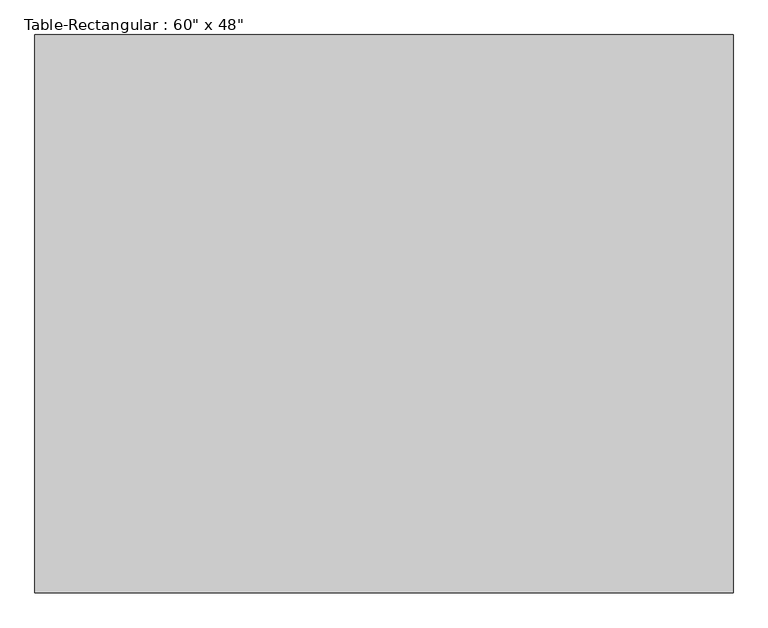
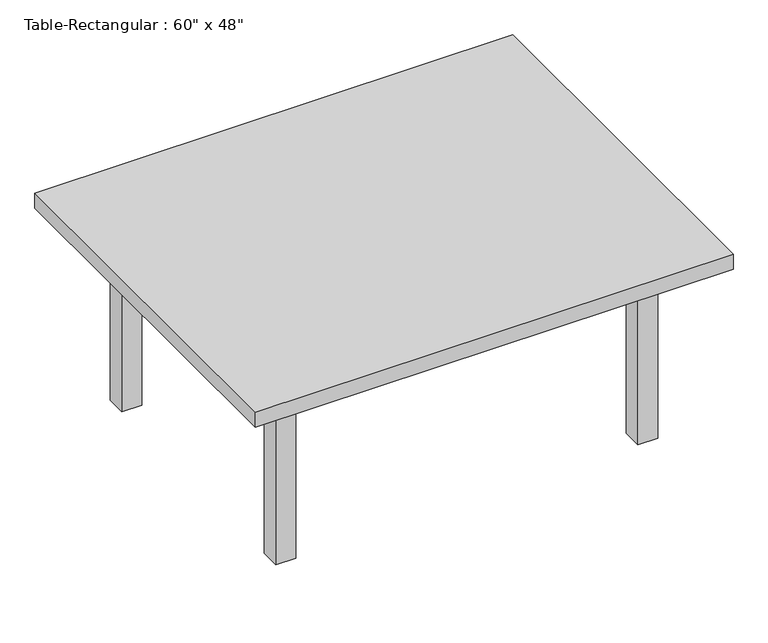
"""IFC4 building model written with IfcOpenShell, lengths in millimetres: furniture geometry."""

from ifc_helpers import new_model, si_unit, frame, origin, origin_with_axes, place, context, project, spatial, polyline, outline, extrude, source, transform, mapped, element, save


def furniture_e8434c74(model_context):
    return source(origin(), model_context, "Body", "SweptSolid", [
        extrude(outline(polyline([(546.1, 419.1), (546.1, 393.7), (-546.1, 393.7), (-546.1, 419.1), (546.1, 419.1)])), frame((0.0, 0.0, 508.0), z_axis=(0.0, 0.0, 1.0), x_axis=(1.0, 0.0, 0.0)), (0.0, 0.0, 1.0), 101.6),
        extrude(outline(polyline([(546.1, -419.1), (-546.1, -419.1), (-546.1, -393.7), (546.1, -393.7), (546.1, -419.1)])), frame((0.0, 0.0, 508.0), z_axis=(0.0, 0.0, 1.0), x_axis=(1.0, 0.0, 0.0)), (0.0, 0.0, 1.0), 101.6),
        extrude(outline(polyline([(-558.8, -393.7), (-584.2, -393.7), (-584.2, 393.7), (-558.8, 393.7), (-558.8, -393.7)])), frame((0.0, 0.0, 508.0), z_axis=(0.0, 0.0, 1.0), x_axis=(1.0, 0.0, 0.0)), (0.0, 0.0, 1.0), 101.6),
        extrude(outline(polyline([(558.8, -393.7), (558.8, 393.7), (584.2, 393.7), (584.2, -393.7), (558.8, -393.7)])), frame((0.0, 0.0, 508.0), z_axis=(0.0, 0.0, 1.0), x_axis=(1.0, 0.0, 0.0)), (0.0, 0.0, 1.0), 101.6),
        extrude(outline(polyline([(762.0, 609.6), (762.0, -609.6), (-762.0, -609.6), (-762.0, 609.6), (762.0, 609.6)])), frame((0.0, 0.0, 609.6), z_axis=(0.0, 0.0, 1.0), x_axis=(1.0, 0.0, 0.0)), (0.0, 0.0, 1.0), 50.8),
        extrude(outline(polyline([(-546.1, 457.2), (-546.1, 393.7), (-609.6, 393.7), (-609.6, 457.2), (-546.1, 457.2)])), origin_with_axes(), (0.0, 0.0, 1.0), 609.6),
        extrude(outline(polyline([(546.1, 457.2), (609.6, 457.2), (609.6, 393.7), (546.1, 393.7), (546.1, 457.2)])), origin_with_axes(), (0.0, 0.0, 1.0), 609.6),
        extrude(outline(polyline([(-546.1, -457.2), (-609.6, -457.2), (-609.6, -393.7), (-546.1, -393.7), (-546.1, -457.2)])), origin_with_axes(), (0.0, 0.0, 1.0), 609.6),
        extrude(outline(polyline([(546.1, -457.2), (546.1, -393.7), (609.6, -393.7), (609.6, -457.2), (546.1, -457.2)])), origin_with_axes(), (0.0, 0.0, 1.0), 609.6),
    ])


if __name__ == "__main__":
    model = new_model("IFC4")
    model_context = context("Model", 3, world=origin())
    ifc_project = project(units=[si_unit("LENGTHUNIT", "METRE", prefix="MILLI")], contexts=[model_context])
    site = spatial("IfcSite", under=ifc_project)
    building = spatial("IfcBuilding", under=site)
    placement = place(None, origin())
    furniture_shape = furniture_e8434c74(model_context)
    element("IfcFurniture", 1, ObjectType="Table-Rectangular : 60\" x 48\"", at=placement, inside=building, context=model_context, shape_type="MappedRepresentation", body=[
        mapped(furniture_shape, transform((0.0, 0.0, 0.0), x_axis=(1.0, 0.0, 0.0), y_axis=(0.0, 1.0, 0.0), z_axis=(0.0, 0.0, 1.0))),
    ])
    save(model, "model.ifc")

# Revit data of these elements
# Type "Table-Rectangular : 60\" x 48\""
#   Assembly Code = "E2020200"
#   Height = 2' - 2"
#   Length = 5' - 0"
#   Width = 4' - 0"
#   Base Material = Birch
#   Top Material = Birch
#   Default Elevation = 0
# Element 1 (IfcFurniture, "Table-Rectangular : 60\" x 48\"")
#   Materials on its faces: "Birch"
# Materials
#   "Birch": class "Wood", colour RGB 224 178 126, transparency 0, Description = "Betula Alleghaniensis", Cost = 0
